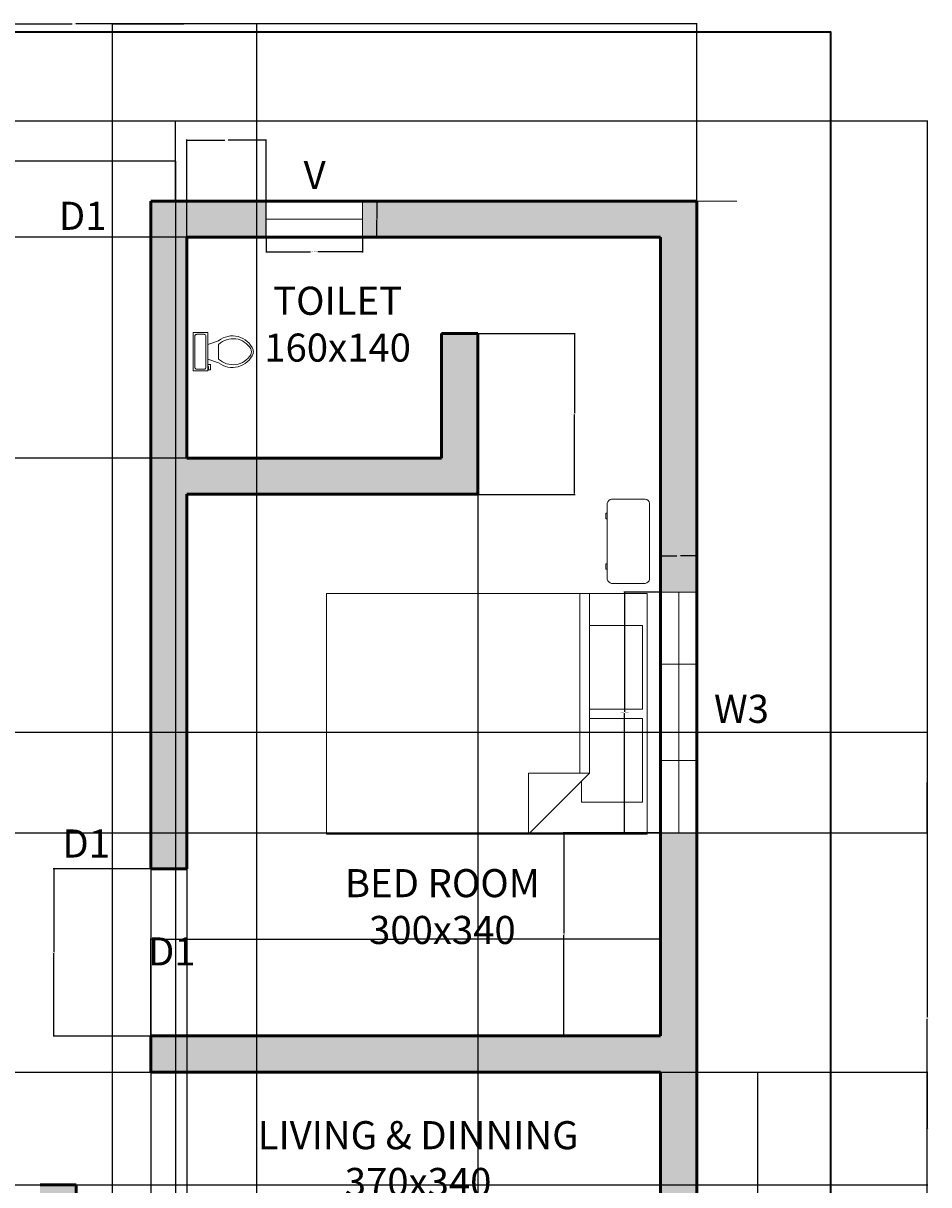
# Model space of a CAD drawing. Units: inches. Extents: x 5191 to 5616, y 7031 to 7539.
# Tile 4 of 4: x 5390 to 5616, y 7250 to 7539. Entities that reach past the tile are written whole.
import ezdxf

# ---------------------------------------------------------------- set-up
doc = ezdxf.new("R2010")
doc.units = ezdxf.units.IN
for name, color, linetype, lineweight in [('A-ANNO-DIMS', 2, 'Continuous', 13), ('A-ANNO-TEXT', 7, 'Continuous', 18), ('A-ANNO-TTLB', 7, 'Continuous', 35), ('A-AREA-IDEN', 7, 'Continuous', 25), ('A-FLOR-FIXT', 9, 'Continuous', 18), ('A-FLOR-STRS', 7, 'Continuous', 25), ('A-FURN', 8, 'Continuous', 18), ('A-GLAZ', 4, 'Continuous', 18), ('A-WALL', 7, 'Continuous', 50)]:
    doc.layers.add(name, color=color, linetype=linetype, lineweight=lineweight)
doc.layers.add('A-WALL-PATT', color=177, linetype='Continuous', lineweight=13, true_color=0x293189)
doc.styles.get("Standard").update_dxf_attribs({"font": 'arial.ttf'})
doc.dimstyles.get("Standard").update_dxf_attribs({"dimtxt": 0.18, "dimasz": 0.18, "dimexe": 0.18, "dimexo": 0.0625, "dimgap": 0.09, "dimtad": 0, "dimtih": 1, "dimtoh": 1, "dimdec": 4, "dimzin": 0, "dimdsep": 46, "dimtxsty": 'Standard', "dimcen": 0.09, "dimadec": 0, "dimazin": 0, "dimtfac": 1, "dimtdec": 4, "dimtofl": 0, "dimtmove": 0, "dimatfit": 3, "dimfxl": 1, "dimtolj": 1, "dimtzin": 0, "dimarcsym": 0})

# ---------------------------------------------------------------- blocks, each defined once
blk = doc.blocks.new('*U2')
for p, q in [((9.5, -6), (9.5, -2)), ((-10, -8.5), (-8, -8.5)), ((-10, -9.5), (-10, -8.5)), ((-7, -9.5), (-10, -9.5)), ((-8, -8.5), (-8, -8)), ((-7, -8), (-7, -9.5)), ((-4, -8), (-6, -14)), ((4, -8), (6, -14)), ((4, -14), (-4, -14))]:
    blk.add_line(p, q)
blk.add_lwpolyline([(10.5, -8), (10.5, 0), (-10.5, 0), (-10.5, -8)], close=True)
for points in [[(-9.5, -2), (-9.5, -6)], [(8.5, -1), (-8.5, -1)], [(-8.5, -7), (8.5, -7)]]:
    blk.add_lwpolyline(points)
for centre, radius, start, end in [((-8.62, -1.88), 0.884, 81.8699, 188.1301), ((-8.62, -6.12), 0.884, 171.8699, 278.1301), ((8.62, -1.88), 0.884, 351.8699, 98.1301), ((8.62, -6.12), 0.884, 261.8699, 8.1301), ((3.52, -21.58), 12.17, 141.46911, 247.97143), ((4.2, -21.82), 11.33, 136.36773, 238.94682), ((-3.52, -21.58), 12.17, 292.02843, 38.53071), ((-4.2, -21.82), 11.33, 301.05301, 43.63209), ((0, -27.88), 4, 245.73182, 294.26817), ((0, -29), 4, 254.86053, 285.13947)]:
    blk.add_arc(centre, radius, start, end)
blk = doc.blocks.new('Bed - Queen')
for p, q in [((0, -80.00003), (0, 0)), ((0, 0), (59.99999, 0)), ((59.99999, 0), (59.99999, -80.00003)), ((7.99999, -1.2), (28.79998, -1.2)), ((7.99999, -14.4), (7.99999, -1.2)), ((28.79998, -1.2), (28.79998, -14.4)), ((31.19999, -1.2), (51.99999, -1.2)), ((31.19999, -14.4), (31.19999, -1.2)), ((51.99999, -1.2), (51.99999, -16.4)), ((0, -14.4), (44.8, -14.4)), ((59.99999, -29.6), (44.8, -14.4)), ((44.8, -14.4), (44.8, -29.6)), ((44.8, -16.8), (0, -16.8)), ((51.99999, -16.4), (46.79936, -16.4)), ((44.8, -29.6), (59.99999, -29.6)), ((59.99999, -80.00003), (0, -80.00003))]:
    blk.add_line(p, q)
blk = doc.blocks.new('Desk - 30 x 60 in.')
for p, q in [((-26.999995, 0), (26.999995, 0)), ((-29.999995, -27), (-29.999995, -3)), ((29.999995, -3), (29.999995, -27)), ((26.999995, -30), (-26.999995, -30)), ((-20.000005, -30), (-20.000005, -31)), ((-20.000005, -31), (-16.000005, -31)), ((-16.000005, -31), (-16.000005, -30)), ((15.999995, -31), (15.999995, -30)), ((19.999995, -31), (15.999995, -31)), ((19.999995, -30), (19.999995, -31))]:
    blk.add_line(p, q)
for centre, start, end in [((-26.499995, -3.5), 98.1301, 171.8699), ((26.499995, -3.5), 8.130102, 81.8699), ((-26.499995, -26.5), 188.1301, 261.8699), ((26.499995, -26.5), 278.1301, 351.8699)]:
    blk.add_arc(centre, 3.535534, start, end)
blk = doc.blocks.new('WIN-W3-60IN')
for p, q in [((9, 60), (0, 60)), ((4.5, 60), (4.5, 0)), ((9, 42), (0, 42)), ((9, 18), (0, 18)), ((9, 0), (0, 0))]:
    blk.add_line(p, q)
blk = doc.blocks.new('VENT-24IN')
for p, q in [((0, 0), (0, 9)), ((24, 0), (24, 9)), ((0, 4.5), (24, 4.5))]:
    blk.add_line(p, q)
blk = doc.blocks.new('*D17')
at = {"layer": 'A-ANNO-DIMS', "color": 0, "lineweight": -2, "transparency": 16777216}
for p, q in [((5549.01, 7397.33), (5539.89, 7397.33)), ((5540.07, 7397.15), (5540.07, 7367.52)), ((5540.07, 7337.51), (5540.07, 7367.15)), ((5549.01, 7337.33), (5539.89, 7337.33))]:
    blk.add_line(p, q, dxfattribs=at)
at = {"layer": 'A-ANNO-DIMS', "color": 0, "transparency": 16777216}
for points in [[(5540.04, 7397.15), (5540.1, 7397.15), (5540.07, 7397.33)], [(5540.04, 7337.51), (5540.1, 7337.51), (5540.07, 7337.33)]]:
    blk.add_solid(points, dxfattribs=at)
at = {"layer": 'Defpoints', "color": 0, "transparency": 16777216}
for p in [(5540.07, 7397.33), (5549.07, 7397.33), (5549.07, 7337.33)]:
    blk.add_point(p, dxfattribs=at)
at = {"layer": 'A-ANNO-DIMS', "color": 0, "transparency": 16777216, "insert": (5540.07, 7367.33), "char_height": 0.18, "attachment_point": 5}
blk.add_mtext('\\A1;WINDOW W3 60 TYP.', dxfattribs=at)
blk = doc.blocks.new('*D18')
at = {"layer": 'A-ANNO-DIMS', "color": 0, "lineweight": -2, "transparency": 16777216}
for p, q in [((5549.07, 7397.4), (5549.07, 7406.51)), ((5549.25, 7406.33), (5553.11, 7406.33)), ((5557.89, 7406.33), (5554.03, 7406.33)), ((5558.07, 7397.4), (5558.07, 7406.51))]:
    blk.add_line(p, q, dxfattribs=at)
at = {"layer": 'A-ANNO-DIMS', "color": 0, "transparency": 16777216}
for points in [[(5549.25, 7406.36), (5549.25, 7406.3), (5549.07, 7406.33)], [(5557.89, 7406.36), (5557.89, 7406.3), (5558.07, 7406.33)]]:
    blk.add_solid(points, dxfattribs=at)
at = {"layer": 'Defpoints', "color": 0, "transparency": 16777216}
for p in [(5558.07, 7406.33), (5549.07, 7397.33), (5558.07, 7397.33)]:
    blk.add_point(p, dxfattribs=at)
at = {"layer": 'A-ANNO-DIMS', "color": 0, "transparency": 16777216, "insert": (5553.57, 7406.33), "char_height": 0.18, "attachment_point": 5}
blk.add_mtext('\\A1;9 TYP.', dxfattribs=at)
blk = doc.blocks.new('*D21')
at = {"layer": 'A-ANNO-DIMS', "color": 0, "lineweight": -2, "transparency": 16777216}
for p, q in [((5450.73, 7485.71), (5450.73, 7481.99)), ((5474.73, 7485.71), (5474.73, 7481.99)), ((5450.91, 7482.17), (5461.83, 7482.17)), ((5474.55, 7482.17), (5463.63, 7482.17))]:
    blk.add_line(p, q, dxfattribs=at)
at = {"layer": 'A-ANNO-DIMS', "color": 0, "transparency": 16777216}
for points in [[(5450.91, 7482.2), (5450.91, 7482.14), (5450.73, 7482.17)], [(5474.55, 7482.2), (5474.55, 7482.14), (5474.73, 7482.17)]]:
    blk.add_solid(points, dxfattribs=at)
at = {"layer": 'Defpoints', "color": 0, "transparency": 16777216}
for p in [(5450.73, 7485.77), (5474.73, 7485.77), (5474.73, 7482.17)]:
    blk.add_point(p, dxfattribs=at)
at = {"layer": 'A-ANNO-DIMS', "color": 0, "transparency": 16777216, "insert": (5462.73, 7482.17), "char_height": 0.18, "attachment_point": 5}
blk.add_mtext('\\A1;VENT 24 TYP.', dxfattribs=at)
blk = doc.blocks.new('*D22')
at = {"layer": 'A-ANNO-DIMS', "color": 0, "lineweight": -2, "transparency": 16777216}
for p, q in [((5474.79, 7494.77), (5478.51, 7494.77)), ((5478.33, 7494.59), (5478.33, 7490.46)), ((5478.33, 7485.95), (5478.33, 7490.09)), ((5474.79, 7485.77), (5478.51, 7485.77))]:
    blk.add_line(p, q, dxfattribs=at)
at = {"layer": 'A-ANNO-DIMS', "color": 0, "transparency": 16777216}
for points in [[(5478.3, 7494.59), (5478.36, 7494.59), (5478.33, 7494.77)], [(5478.3, 7485.95), (5478.36, 7485.95), (5478.33, 7485.77)]]:
    blk.add_solid(points, dxfattribs=at)
at = {"layer": 'Defpoints', "color": 0, "transparency": 16777216}
for p in [(5474.73, 7494.77), (5478.33, 7494.77), (5474.73, 7485.77)]:
    blk.add_point(p, dxfattribs=at)
at = {"layer": 'A-ANNO-DIMS', "color": 0, "transparency": 16777216, "insert": (5478.33, 7490.27), "char_height": 0.18, "attachment_point": 5}
blk.add_mtext('\\A1;9 TYP.', dxfattribs=at)
blk = doc.blocks.new('*D31')
at = {"layer": 'A-ANNO-DIMS', "color": 0, "lineweight": -2, "transparency": 16777216}
for p, q in [((5247.63, 7494.84), (5247.63, 7539.1)), ((5247.81, 7538.92), (5402.39, 7538.92)), ((5557.89, 7538.92), (5403.31, 7538.92)), ((5558.07, 7494.84), (5558.07, 7539.1))]:
    blk.add_line(p, q, dxfattribs=at)
at = {"layer": 'A-ANNO-DIMS', "color": 0, "transparency": 16777216}
for points in [[(5247.81, 7538.95), (5247.81, 7538.89), (5247.63, 7538.92)], [(5557.89, 7538.95), (5557.89, 7538.89), (5558.07, 7538.92)]]:
    blk.add_solid(points, dxfattribs=at)
at = {"layer": 'Defpoints', "color": 0, "transparency": 16777216}
for p in [(5558.07, 7538.92), (5247.63, 7494.77), (5558.07, 7494.77)]:
    blk.add_point(p, dxfattribs=at)
at = {"layer": 'A-ANNO-DIMS', "color": 0, "transparency": 16777216, "insert": (5402.85, 7538.92), "char_height": 0.18, "attachment_point": 5}
blk.add_mtext('\\A1;310.44', dxfattribs=at)
blk = doc.blocks.new('*D32')
at = {"layer": 'A-ANNO-DIMS', "color": 0, "lineweight": -2, "transparency": 16777216}
for p, q in [((5428.24, 7514.77), (5615.71, 7514.77)), ((5615.53, 7514.59), (5615.53, 7291.37)), ((5615.53, 7067.79), (5615.53, 7291.01)), ((5466.73, 7067.61), (5615.71, 7067.61))]:
    blk.add_line(p, q, dxfattribs=at)
at = {"layer": 'A-ANNO-DIMS', "color": 0, "transparency": 16777216}
for points in [[(5615.5, 7514.59), (5615.56, 7514.59), (5615.53, 7514.77)], [(5615.5, 7067.79), (5615.56, 7067.79), (5615.53, 7067.61)]]:
    blk.add_solid(points, dxfattribs=at)
at = {"layer": 'Defpoints', "color": 0, "transparency": 16777216}
for p in [(5428.18, 7514.77), (5615.53, 7514.77), (5466.67, 7067.61)]:
    blk.add_point(p, dxfattribs=at)
at = {"layer": 'A-ANNO-DIMS', "color": 0, "transparency": 16777216, "insert": (5615.53, 7291.19), "char_height": 0.18, "attachment_point": 5}
blk.add_mtext('\\A1;447.2', dxfattribs=at)
blk = doc.blocks.new('*D38')
at = {"layer": 'A-ANNO-DIMS', "color": 0, "lineweight": -2, "transparency": 16777216}
for p, q in [((5379.71, 7504.71), (5379.71, 7030.92)), ((5428.18, 7504.71), (5428.18, 7030.92)), ((5379.89, 7031.1), (5403.55, 7031.1)), ((5428, 7031.1), (5404.34, 7031.1))]:
    blk.add_line(p, q, dxfattribs=at)
at = {"layer": 'A-ANNO-DIMS', "color": 0, "transparency": 16777216}
for points in [[(5379.89, 7031.13), (5379.89, 7031.07), (5379.71, 7031.1)], [(5428, 7031.13), (5428, 7031.07), (5428.18, 7031.1)]]:
    blk.add_solid(points, dxfattribs=at)
at = {"layer": 'Defpoints', "color": 0, "transparency": 16777216}
for p in [(5379.71, 7504.77), (5428.18, 7504.77), (5428.18, 7031.1)]:
    blk.add_point(p, dxfattribs=at)
at = {"layer": 'A-ANNO-DIMS', "color": 0, "transparency": 16777216, "insert": (5403.95, 7031.1), "char_height": 0.18, "attachment_point": 5}
blk.add_mtext('\\A1;48.47', dxfattribs=at)
blk = doc.blocks.new('*D44')
at = {"layer": 'A-ANNO-DIMS', "color": 0, "lineweight": -2, "transparency": 16777216}
for p, q in [((5549.13, 7277.69), (5573.4, 7277.69)), ((5573.22, 7277.51), (5573.22, 7210.98)), ((5573.22, 7144.07), (5573.22, 7210.61)), ((5549.13, 7143.89), (5573.4, 7143.89))]:
    blk.add_line(p, q, dxfattribs=at)
at = {"layer": 'A-ANNO-DIMS', "color": 0, "transparency": 16777216}
for points in [[(5573.19, 7277.51), (5573.25, 7277.51), (5573.22, 7277.69)], [(5573.19, 7144.07), (5573.25, 7144.07), (5573.22, 7143.89)]]:
    blk.add_solid(points, dxfattribs=at)
at = {"layer": 'Defpoints', "color": 0, "transparency": 16777216}
for p in [(5549.07, 7277.69), (5549.07, 7143.89), (5573.22, 7143.89)]:
    blk.add_point(p, dxfattribs=at)
at = {"layer": 'A-ANNO-DIMS', "color": 0, "transparency": 16777216, "insert": (5573.22, 7210.79), "char_height": 0.18, "attachment_point": 5}
blk.add_mtext('\\A1;133.8', dxfattribs=at)
blk = doc.blocks.new('*D45')
at = {"layer": 'A-ANNO-DIMS', "color": 0, "lineweight": -2, "transparency": 16777216}
for p, q in [((5421.99, 7286.76), (5421.99, 7311.02)), ((5422.17, 7310.84), (5485.08, 7310.84)), ((5548.89, 7310.84), (5485.99, 7310.84)), ((5549.07, 7286.76), (5549.07, 7311.02))]:
    blk.add_line(p, q, dxfattribs=at)
at = {"layer": 'A-ANNO-DIMS', "color": 0, "transparency": 16777216}
for points in [[(5422.17, 7310.87), (5422.17, 7310.81), (5421.99, 7310.84)], [(5548.89, 7310.87), (5548.89, 7310.81), (5549.07, 7310.84)]]:
    blk.add_solid(points, dxfattribs=at)
at = {"layer": 'Defpoints', "color": 0, "transparency": 16777216}
for p in [(5549.07, 7310.84), (5421.99, 7286.69), (5549.07, 7286.69)]:
    blk.add_point(p, dxfattribs=at)
at = {"layer": 'A-ANNO-DIMS', "color": 0, "transparency": 16777216, "insert": (5485.53, 7310.84), "char_height": 0.18, "attachment_point": 5}
blk.add_mtext('\\A1;127.08', dxfattribs=at)
blk = doc.blocks.new('*D46')
at = {"layer": 'A-ANNO-DIMS', "color": 0, "lineweight": -2, "transparency": 16777216}
for p, q in [((5549.01, 7337.33), (5524.74, 7337.33)), ((5524.92, 7337.15), (5524.92, 7312.2)), ((5524.92, 7286.87), (5524.92, 7311.83)), ((5549.01, 7286.69), (5524.74, 7286.69))]:
    blk.add_line(p, q, dxfattribs=at)
at = {"layer": 'A-ANNO-DIMS', "color": 0, "transparency": 16777216}
for points in [[(5524.89, 7337.15), (5524.95, 7337.15), (5524.92, 7337.33)], [(5524.89, 7286.87), (5524.95, 7286.87), (5524.92, 7286.69)]]:
    blk.add_solid(points, dxfattribs=at)
at = {"layer": 'Defpoints', "color": 0, "transparency": 16777216}
for p in [(5524.92, 7337.33), (5549.07, 7337.33), (5549.07, 7286.69)]:
    blk.add_point(p, dxfattribs=at)
at = {"layer": 'A-ANNO-DIMS', "color": 0, "transparency": 16777216, "insert": (5524.92, 7312.01), "char_height": 0.18, "attachment_point": 5}
blk.add_mtext('\\A1;50.64', dxfattribs=at)
blk = doc.blocks.new('*D49')
at = {"layer": 'A-ANNO-DIMS', "color": 0, "lineweight": -2, "transparency": 16777216}
for p, q in [((5385.99, 7494.71), (5385.99, 7030.92)), ((5421.99, 7494.71), (5421.99, 7030.92)), ((5386.17, 7031.1), (5403.77, 7031.1)), ((5421.81, 7031.1), (5404.21, 7031.1))]:
    blk.add_line(p, q, dxfattribs=at)
at = {"layer": 'A-ANNO-DIMS', "color": 0, "transparency": 16777216}
for points in [[(5386.17, 7031.13), (5386.17, 7031.07), (5385.99, 7031.1)], [(5421.81, 7031.13), (5421.81, 7031.07), (5421.99, 7031.1)]]:
    blk.add_solid(points, dxfattribs=at)
at = {"layer": 'Defpoints', "color": 0, "transparency": 16777216}
for p in [(5385.99, 7494.77), (5421.99, 7494.77), (5421.99, 7031.1)]:
    blk.add_point(p, dxfattribs=at)
at = {"layer": 'A-ANNO-DIMS', "color": 0, "transparency": 16777216, "insert": (5403.99, 7031.1), "char_height": 0.18, "attachment_point": 5}
blk.add_mtext('\\A1;36', dxfattribs=at)
blk = doc.blocks.new('*D50')
at = {"layer": 'A-ANNO-DIMS', "color": 0, "lineweight": -2, "transparency": 16777216}
for p, q in [((5430.99, 7485.84), (5430.99, 7510.1)), ((5431.17, 7509.92), (5440.48, 7509.92)), ((5450.55, 7509.92), (5441.25, 7509.92)), ((5450.73, 7485.84), (5450.73, 7510.1))]:
    blk.add_line(p, q, dxfattribs=at)
at = {"layer": 'A-ANNO-DIMS', "color": 0, "transparency": 16777216}
for points in [[(5431.17, 7509.95), (5431.17, 7509.89), (5430.99, 7509.92)], [(5450.55, 7509.95), (5450.55, 7509.89), (5450.73, 7509.92)]]:
    blk.add_solid(points, dxfattribs=at)
at = {"layer": 'Defpoints', "color": 0, "transparency": 16777216}
for p in [(5450.73, 7509.92), (5430.99, 7485.77), (5450.73, 7485.77)]:
    blk.add_point(p, dxfattribs=at)
at = {"layer": 'A-ANNO-DIMS', "color": 0, "transparency": 16777216, "insert": (5440.86, 7509.92), "char_height": 0.18, "attachment_point": 5}
blk.add_mtext('\\A1;19.74', dxfattribs=at)
blk = doc.blocks.new('*D51')
at = {"layer": 'A-ANNO-DIMS', "color": 0, "lineweight": -2, "transparency": 16777216}
for p, q in [((5412.46, 7143.96), (5412.46, 7539.1)), ((5412.64, 7538.92), (5430.24, 7538.92)), ((5448.28, 7538.92), (5430.68, 7538.92)), ((5448.46, 7143.96), (5448.46, 7539.1))]:
    blk.add_line(p, q, dxfattribs=at)
at = {"layer": 'A-ANNO-DIMS', "color": 0, "transparency": 16777216}
for points in [[(5412.64, 7538.95), (5412.64, 7538.89), (5412.46, 7538.92)], [(5448.28, 7538.95), (5448.28, 7538.89), (5448.46, 7538.92)]]:
    blk.add_solid(points, dxfattribs=at)
at = {"layer": 'Defpoints', "color": 0, "transparency": 16777216}
for p in [(5448.46, 7538.92), (5412.46, 7143.89), (5448.46, 7143.89)]:
    blk.add_point(p, dxfattribs=at)
at = {"layer": 'A-ANNO-DIMS', "color": 0, "transparency": 16777216, "insert": (5430.46, 7538.92), "char_height": 0.18, "attachment_point": 5}
blk.add_mtext('\\A1;36', dxfattribs=at)
blk = doc.blocks.new('*D54')
at = {"layer": 'A-ANNO-DIMS', "color": 0, "lineweight": -2, "transparency": 16777216}
for p, q in [((5430.99, 7421.63), (5430.99, 7030.92)), ((5503.47, 7421.63), (5503.47, 7030.92)), ((5431.17, 7031.1), (5466.84, 7031.1)), ((5503.29, 7031.1), (5467.62, 7031.1))]:
    blk.add_line(p, q, dxfattribs=at)
at = {"layer": 'A-ANNO-DIMS', "color": 0, "transparency": 16777216}
for points in [[(5431.17, 7031.13), (5431.17, 7031.07), (5430.99, 7031.1)], [(5503.29, 7031.13), (5503.29, 7031.07), (5503.47, 7031.1)]]:
    blk.add_solid(points, dxfattribs=at)
at = {"layer": 'Defpoints', "color": 0, "transparency": 16777216}
for p in [(5430.99, 7421.69), (5503.47, 7421.69), (5503.47, 7031.1)]:
    blk.add_point(p, dxfattribs=at)
at = {"layer": 'A-ANNO-DIMS', "color": 0, "transparency": 16777216, "insert": (5467.23, 7031.1), "char_height": 0.18, "attachment_point": 5}
blk.add_mtext('\\A1;72.48', dxfattribs=at)
blk = doc.blocks.new('*D55')
at = {"layer": 'A-ANNO-DIMS', "color": 0, "lineweight": -2, "transparency": 16777216}
for p, q in [((5430.93, 7485.77), (5191.41, 7485.77)), ((5191.59, 7485.59), (5191.59, 7458.42)), ((5191.59, 7430.87), (5191.59, 7458.05)), ((5430.93, 7430.69), (5191.41, 7430.69))]:
    blk.add_line(p, q, dxfattribs=at)
at = {"layer": 'A-ANNO-DIMS', "color": 0, "transparency": 16777216}
for points in [[(5191.56, 7485.59), (5191.62, 7485.59), (5191.59, 7485.77)], [(5191.56, 7430.87), (5191.62, 7430.87), (5191.59, 7430.69)]]:
    blk.add_solid(points, dxfattribs=at)
at = {"layer": 'Defpoints', "color": 0, "transparency": 16777216}
for p in [(5191.59, 7485.77), (5430.99, 7485.77), (5430.99, 7430.69)]:
    blk.add_point(p, dxfattribs=at)
at = {"layer": 'A-ANNO-DIMS', "color": 0, "transparency": 16777216, "insert": (5191.59, 7458.23), "char_height": 0.18, "attachment_point": 5}
blk.add_mtext('\\A1;55.08', dxfattribs=at)
blk = doc.blocks.new('*D60')
at = {"layer": 'A-ANNO-DIMS', "color": 0, "lineweight": -2, "transparency": 16777216}
for p, q in [((5343.97, 7277.69), (5615.71, 7277.69)), ((5615.53, 7277.51), (5615.53, 7263.84)), ((5615.53, 7249.79), (5615.53, 7263.47)), ((5343.97, 7249.61), (5615.71, 7249.61))]:
    blk.add_line(p, q, dxfattribs=at)
at = {"layer": 'A-ANNO-DIMS', "color": 0, "transparency": 16777216}
for points in [[(5615.5, 7277.51), (5615.56, 7277.51), (5615.53, 7277.69)], [(5615.5, 7249.79), (5615.56, 7249.79), (5615.53, 7249.61)]]:
    blk.add_solid(points, dxfattribs=at)
at = {"layer": 'Defpoints', "color": 0, "transparency": 16777216}
for p in [(5343.91, 7277.69), (5615.53, 7277.69), (5343.91, 7249.61)]:
    blk.add_point(p, dxfattribs=at)
at = {"layer": 'A-ANNO-DIMS', "color": 0, "transparency": 16777216, "insert": (5615.53, 7263.65), "char_height": 0.18, "attachment_point": 5}
blk.add_mtext('\\A1;28.08', dxfattribs=at)
blk = doc.blocks.new('*D62')
at = {"layer": 'A-ANNO-DIMS', "color": 0, "lineweight": -2, "transparency": 16777216}
for p, q in [((5361.85, 7362.43), (5615.71, 7362.43)), ((5615.53, 7362.25), (5615.53, 7350.06)), ((5615.53, 7337.51), (5615.53, 7349.7)), ((5361.85, 7337.33), (5615.71, 7337.33))]:
    blk.add_line(p, q, dxfattribs=at)
at = {"layer": 'A-ANNO-DIMS', "color": 0, "transparency": 16777216}
for points in [[(5615.5, 7362.25), (5615.56, 7362.25), (5615.53, 7362.43)], [(5615.5, 7337.51), (5615.56, 7337.51), (5615.53, 7337.33)]]:
    blk.add_solid(points, dxfattribs=at)
at = {"layer": 'Defpoints', "color": 0, "transparency": 16777216}
for p in [(5361.78, 7362.43), (5615.53, 7362.43), (5361.78, 7337.33)]:
    blk.add_point(p, dxfattribs=at)
at = {"layer": 'A-ANNO-DIMS', "color": 0, "transparency": 16777216, "insert": (5615.53, 7349.88), "char_height": 0.18, "attachment_point": 5}
blk.add_mtext('\\A1;25.094', dxfattribs=at)
blk = doc.blocks.new('*D65')
at = {"layer": 'A-ANNO-DIMS', "color": 0, "lineweight": -2, "transparency": 16777216}
for p, q in [((5421.93, 7328.33), (5397.66, 7328.33)), ((5397.84, 7328.15), (5397.84, 7307.7)), ((5397.84, 7286.87), (5397.84, 7307.33)), ((5421.93, 7286.69), (5397.66, 7286.69))]:
    blk.add_line(p, q, dxfattribs=at)
at = {"layer": 'A-ANNO-DIMS', "color": 0, "transparency": 16777216}
for points in [[(5397.81, 7328.15), (5397.87, 7328.15), (5397.84, 7328.33)], [(5397.81, 7286.87), (5397.87, 7286.87), (5397.84, 7286.69)]]:
    blk.add_solid(points, dxfattribs=at)
at = {"layer": 'Defpoints', "color": 0, "transparency": 16777216}
for p in [(5397.84, 7328.33), (5421.99, 7328.33), (5421.99, 7286.69)]:
    blk.add_point(p, dxfattribs=at)
at = {"layer": 'A-ANNO-DIMS', "color": 0, "transparency": 16777216, "insert": (5397.84, 7307.51), "char_height": 0.18, "attachment_point": 5}
blk.add_mtext('\\A1;41.64', dxfattribs=at)
blk = doc.blocks.new('*D66')
at = {"layer": 'A-ANNO-DIMS', "color": 0, "lineweight": -2, "transparency": 16777216}
for p, q in [((5503.53, 7461.77), (5527.8, 7461.77)), ((5527.62, 7461.59), (5527.62, 7441.92)), ((5527.62, 7421.87), (5527.62, 7441.55)), ((5503.53, 7421.69), (5527.8, 7421.69))]:
    blk.add_line(p, q, dxfattribs=at)
at = {"layer": 'A-ANNO-DIMS', "color": 0, "transparency": 16777216}
for points in [[(5527.59, 7461.59), (5527.65, 7461.59), (5527.62, 7461.77)], [(5527.59, 7421.87), (5527.65, 7421.87), (5527.62, 7421.69)]]:
    blk.add_solid(points, dxfattribs=at)
at = {"layer": 'Defpoints', "color": 0, "transparency": 16777216}
for p in [(5503.47, 7461.77), (5503.47, 7421.69), (5527.62, 7421.69)]:
    blk.add_point(p, dxfattribs=at)
at = {"layer": 'A-ANNO-DIMS', "color": 0, "transparency": 16777216, "insert": (5527.62, 7441.73), "char_height": 0.18, "attachment_point": 5}
blk.add_mtext('\\A1;40.08', dxfattribs=at)

msp = doc.modelspace()

# ---------------------------------------------------------------- hatches: boundary and pattern name
at = {"layer": 'A-WALL-PATT'}
h = msp.add_hatch(color=256, dxfattribs=at)
h.dxf.hatch_style = 1
h.paths.add_polyline_path([(5297.311, 7494.7733), (5247.631, 7494.7733), (5247.631, 7441.5533), (5256.631, 7441.5533), (5256.631, 7485.7733), (5297.311, 7485.7733)])
h.paths.add_polyline_path([(5503.471, 7430.6933), (5503.471, 7461.7733), (5494.471, 7461.7733), (5494.471, 7430.6933), (5430.991, 7430.6933), (5430.991, 7485.7733), (5450.731, 7485.7733), (5450.731, 7494.7733), (5421.991, 7494.7733), (5421.991, 7485.7733), (5421.991, 7337.3333), (5421.991, 7328.3333), (5430.991, 7328.3333), (5430.991, 7337.3333), (5430.991, 7421.6933), (5503.471, 7421.6933)])
h.paths.add_polyline_path([(5385.991, 7494.7733), (5345.311, 7494.7733), (5345.311, 7485.7733), (5385.991, 7485.7733)])
h.paths.add_polyline_path([(5558.071, 7494.7733), (5474.731, 7494.7733), (5474.731, 7485.7733), (5494.471, 7485.7733), (5503.471, 7485.7733), (5549.071, 7485.7733), (5549.071, 7397.3333), (5558.071, 7397.3333)])
h.paths.add_polyline_path([(5385.991, 7337.3333), (5256.631, 7337.3333), (5256.631, 7381.5533), (5247.631, 7381.5533), (5247.631, 7337.3333), (5247.631, 7328.3333), (5247.631, 7300.9733), (5256.631, 7300.9733), (5256.631, 7328.3333), (5385.991, 7328.3333)])
h.paths.add_polyline_path([(5358.391, 7249.6133), (5303.911, 7249.6133), (5256.631, 7249.6133), (5256.631, 7276.9733), (5247.631, 7276.9733), (5247.631, 7249.6133), (5247.631, 7240.6133), (5247.631, 7207.6133), (5256.631, 7207.6133), (5256.631, 7240.6133), (5303.911, 7240.6133), (5358.391, 7240.6133)])
h.paths.add_polyline_path([(5256.631, 7114.6133), (5256.631, 7147.6133), (5247.631, 7147.6133), (5247.631, 7114.6133), (5247.631, 7105.6133), (5247.631, 7087.6133), (5301.511, 7087.6133), (5301.511, 7096.6133), (5256.631, 7096.6133)])
h.paths.add_polyline_path([(5403.391, 7105.6133), (5403.391, 7114.6133), (5403.391, 7134.8933), (5412.4598, 7134.8933), (5412.4598, 7143.8933), (5403.391, 7143.8933), (5403.391, 7249.6133), (5394.391, 7249.6133), (5394.391, 7143.8933), (5394.391, 7134.8933), (5394.391, 7114.6133), (5394.391, 7096.6133), (5349.511, 7096.6133), (5349.511, 7087.6133), (5403.391, 7087.6133)])
h.paths.add_polyline_path([(5558.071, 7143.8933), (5558.071, 7186.7933), (5549.071, 7186.7933), (5549.071, 7143.8933), (5527.2654, 7143.8933), (5527.2654, 7134.8933), (5558.071, 7134.8933)])
h.paths.add_polyline_path([(5479.2654, 7143.8933), (5448.4598, 7143.8933), (5448.4598, 7134.8933), (5479.2654, 7134.8933)])
h.paths.add_polyline_path([(5558.071, 7337.3333), (5549.071, 7337.3333), (5549.071, 7286.6933), (5421.991, 7286.6933), (5421.991, 7277.6933), (5430.991, 7277.6933), (5549.071, 7277.6933), (5549.071, 7234.7933), (5558.071, 7234.7933), (5558.071, 7277.6933)])

# ---------------------------------------------------------------- linework, layer by layer
at = {"layer": 'A-ANNO-DIMS'}
for q in [(5558.071, 7504.7733), (5568.071, 7494.7733)]:
    msp.add_line((5558.071, 7494.7733), q, dxfattribs=at)
at = {"layer": 'A-ANNO-TTLB'}
msp.add_lwpolyline([(5215.7388, 7536.9841), (5591.3795, 7536.9841), (5591.3795, 7055.2452), (5215.7388, 7055.2452)], close=True, dxfattribs=at)
at = {"layer": 'A-FLOR-STRS'}
for p, q in [((5379.7136, 7514.7733), (5428.1805, 7514.7733)), ((5428.1805, 7494.7733), (5428.1805, 7514.7733)), ((5379.7136, 7504.7733), (5428.1805, 7504.7733))]:
    msp.add_line(p, q, dxfattribs=at)
at = {"layer": 'A-GLAZ'}
msp.add_line((5549.071, 7397.3333), (5549.071, 7337.3333), dxfattribs=at)
at = {"layer": 'A-WALL'}
for p, q in [((5421.991, 7485.7733), (5421.991, 7494.7733)), ((5421.991, 7494.7733), (5558.071, 7494.7733)), ((5558.071, 7494.7733), (5558.071, 7337.3333)), ((5421.991, 7485.7733), (5421.991, 7337.3333)), ((5430.991, 7485.7733), (5430.991, 7430.6933)), ((5430.991, 7485.7733), (5494.471, 7485.7733)), ((5494.471, 7485.7733), (5503.471, 7485.7733)), ((5503.471, 7485.7733), (5549.071, 7485.7733)), ((5549.071, 7485.7733), (5549.071, 7337.3333)), ((5494.471, 7461.7733), (5494.471, 7430.6933)), ((5494.471, 7461.7733), (5503.471, 7461.7733)), ((5503.471, 7461.7733), (5503.471, 7430.6933)), ((5430.991, 7430.6933), (5494.471, 7430.6933)), ((5503.471, 7430.6933), (5503.471, 7421.6933)), ((5430.991, 7421.6933), (5503.471, 7421.6933)), ((5430.991, 7421.6933), (5430.991, 7337.3333)), ((5421.991, 7337.3333), (5421.991, 7328.3333)), ((5430.991, 7337.3333), (5430.991, 7328.3333)), ((5549.071, 7337.3333), (5549.071, 7286.6933)), ((5558.071, 7337.3333), (5558.071, 7277.6933)), ((5421.991, 7328.3333), (5430.991, 7328.3333)), ((5421.991, 7286.6933), (5549.071, 7286.6933)), ((5421.991, 7286.6933), (5421.991, 7277.6933)), ((5430.991, 7277.6933), (5421.991, 7277.6933)), ((5430.991, 7277.6933), (5549.071, 7277.6933)), ((5549.071, 7277.6933), (5549.071, 7143.8933)), ((5558.071, 7277.6933), (5558.071, 7143.8933)), ((5394.391, 7249.6133), (5403.391, 7249.6133)), ((5403.391, 7249.6133), (5403.391, 7143.8933))]:
    msp.add_line(p, q, dxfattribs=at)

# ---------------------------------------------------------------- block references
at = {"layer": 'A-FLOR-FIXT', "xscale": 0.4558429364465041, "yscale": 0.4558429364465041, "zscale": 0.4558429364465041, "rotation": 90}
msp.add_blockref('*U2', (5432.5183, 7457.2373), dxfattribs=at)
at = {"layer": 'A-FURN', "xscale": 0.350301795417789, "yscale": 0.350301795417789, "zscale": 0.350301795417789, "rotation": 270}
msp.add_blockref('Desk - 30 x 60 in.', (5546.2909, 7410.0149), dxfattribs=at)
at = {"layer": 'A-FURN', "rotation": 270}
msp.add_blockref('Bed - Queen', (5545.7485, 7396.9827), dxfattribs=at)
at = {"layer": 'A-GLAZ'}
for name, p in [('VENT-24IN', (5450.731, 7485.773)), ('WIN-W3-60IN', (5549.071, 7337.333))]:
    msp.add_blockref(name, p, dxfattribs=at)

# ---------------------------------------------------------------- texts
at = {"layer": 'A-ANNO-TEXT', "char_height": 7, "attachment_point": 1}
for s, width, insert in [('\\pxqc;V', 29.703042, (5447.9778, 7504.7663)), ('\\pxqc;D1', 16.947643, (5396.5294, 7494.6114)), ('\\pxqc;W3', 29.703042, (5554.3709, 7371.7303)), ('\\pxqc;D1', 18.543886, (5396.6224, 7338.166)), ('\\pxqc;D1', 18.543886, (5417.9596, 7311.2676))]:
    msp.add_mtext_dynamic_manual_height_columns(s, width=width, gutter_width=12.5, heights=[0], dxfattribs=dict(at, insert=insert))
at = {"layer": 'A-AREA-IDEN', "char_height": 7, "attachment_point": 1}
for s, width, insert in [('\\pxqc;{\\fArial|b1|i0|c0|p34;TOILET\\P160x140}', 45.986288, (5445.562, 7473.4317)), ('\\pxqc;{\\fArial|b1|i0|c0|p34;BED ROOM\\P300x340}', 84.025987, (5452.6555, 7328.2856)), ('\\pxqc;{\\fArial|b1|i0|c0|p34;LIVING & DINNING\\P370x340}', 103.767041, (5436.7343, 7265.4722))]:
    msp.add_mtext_dynamic_manual_height_columns(s, width=width, gutter_width=12.5, heights=[0], dxfattribs=dict(at, insert=insert))

# ---------------------------------------------------------------- dimensions: what is measured, and where the dimension line sits
at = {"layer": 'A-ANNO-DIMS'}
for base, p1, p2, override, picture, middle in [((5558.071, 7538.9233), (5247.631, 7494.7733), (5558.071, 7494.7733), {"dimdec": 2, "dimlfac": 1, "dimrnd": 0, "dimzin": 0, "dimdsep": 46, "dimlunit": 2}, '*D31', (5402.851, 7538.9233)), ((5448.4598, 7538.9233), (5412.4598, 7143.8933), (5448.4598, 7143.8933), {"dimdec": 0, "dimlfac": 1, "dimrnd": 0, "dimzin": 0, "dimdsep": 46, "dimlunit": 2}, '*D51', (5430.4598, 7538.9233)), ((5428.1805, 7031.0952), (5379.7136, 7504.7733), (5428.1805, 7504.7733), {"dimdec": 2, "dimlfac": 1, "dimrnd": 0, "dimzin": 0, "dimdsep": 46, "dimlunit": 2}, '*D38', (5403.947, 7031.0952)), ((5421.991, 7031.0952), (5385.991, 7494.7733), (5421.991, 7494.7733), {"dimdec": 0, "dimlfac": 1, "dimrnd": 0, "dimzin": 0, "dimdsep": 46, "dimlunit": 2}, '*D49', (5403.991, 7031.0952)), ((5503.471, 7031.0952), (5430.991, 7421.6933), (5503.471, 7421.6933), {"dimdec": 2, "dimlfac": 1, "dimrnd": 0, "dimzin": 0, "dimdsep": 46, "dimlunit": 2}, '*D54', (5467.231, 7031.0952))]:
    dim = msp.add_linear_dim(base=base, p1=p1, p2=p2, dimstyle='Standard', override=override, dxfattribs=at)
    dim.commit()
    dim.dimension.update_dxf_attribs({"geometry": picture, "text_midpoint": middle})
for base, p1, p2, angle, override, picture, middle in [((5615.5295, 7514.7733), (5466.6673, 7067.6133), (5428.1805, 7514.7733), 90, {"dimdec": 1, "dimlfac": 1, "dimrnd": 0, "dimzin": 0, "dimdsep": 46, "dimlunit": 2}, '*D32', (5615.5295, 7291.1933)), ((5450.731, 7509.9233), (5430.991, 7485.7733), (5450.731, 7485.7733), 0, {"dimdec": 2, "dimlfac": 1, "dimrnd": 0, "dimzin": 0, "dimdsep": 46, "dimlunit": 2}, '*D50', (5440.861, 7509.9233)), ((5191.5888, 7485.7733), (5430.991, 7430.6933), (5430.991, 7485.7733), 90, {"dimdec": 2, "dimlfac": 1, "dimrnd": 0, "dimzin": 0, "dimdsep": 46, "dimlunit": 2}, '*D55', (5191.5888, 7458.2333)), ((5527.621, 7421.6933), (5503.471, 7461.7733), (5503.471, 7421.6933), 270, {"dimdec": 2, "dimlfac": 1, "dimrnd": 0, "dimzin": 0, "dimdsep": 46, "dimlunit": 2}, '*D66', (5527.621, 7441.7333)), ((5615.5295, 7362.4276), (5361.7831, 7337.3333), (5361.7831, 7362.4276), 90, {"dimdec": 3, "dimlfac": 1, "dimrnd": 0, "dimzin": 0, "dimdsep": 46, "dimlunit": 2}, '*D62', (5615.5295, 7349.8805)), ((5524.921, 7337.3333), (5549.071, 7286.6933), (5549.071, 7337.3333), 90, {"dimdec": 2, "dimlfac": 1, "dimrnd": 0, "dimzin": 0, "dimdsep": 46, "dimlunit": 2}, '*D46', (5524.921, 7312.0133)), ((5397.841, 7328.3333), (5421.991, 7286.6933), (5421.991, 7328.3333), 90, {"dimdec": 2, "dimlfac": 1, "dimrnd": 0, "dimzin": 0, "dimdsep": 46, "dimlunit": 2}, '*D65', (5397.841, 7307.5133)), ((5549.071, 7310.8433), (5421.991, 7286.6933), (5549.071, 7286.6933), 0, {"dimdec": 2, "dimlfac": 1, "dimrnd": 0, "dimzin": 0, "dimdsep": 46, "dimlunit": 2}, '*D45', (5485.531, 7310.8433)), ((5615.5295, 7277.6933), (5343.911, 7249.6133), (5343.911, 7277.6933), 90, {"dimdec": 2, "dimlfac": 1, "dimrnd": 0, "dimzin": 0, "dimdsep": 46, "dimlunit": 2}, '*D60', (5615.5295, 7263.6533)), ((5573.221, 7143.8933), (5549.071, 7277.6933), (5549.071, 7143.8933), 270, {"dimdec": 1, "dimlfac": 1, "dimrnd": 0, "dimzin": 0, "dimdsep": 46, "dimlunit": 2}, '*D44', (5573.221, 7210.7933))]:
    dim = msp.add_linear_dim(base=base, p1=p1, p2=p2, angle=angle, dimstyle='Standard', override=override, dxfattribs=at)
    dim.commit()
    dim.dimension.update_dxf_attribs({"geometry": picture, "text_midpoint": middle})
for base, p1, p2, text, picture, middle in [((5478.331, 7494.7733), (5474.731, 7485.7733), (5474.731, 7494.7733), '<> TYP.', '*D22', (5478.331, 7490.2733)), ((5540.071, 7397.3333), (5549.071, 7337.3333), (5549.071, 7397.3333), 'WINDOW W3 <> TYP.', '*D17', (5540.071, 7367.3333))]:
    dim = msp.add_linear_dim(base=base, p1=p1, p2=p2, angle=90, text=text, dimstyle='Standard', override={"dimdec": 0, "dimlfac": 1, "dimrnd": 0, "dimzin": 0, "dimdsep": 46, "dimlunit": 2}, dxfattribs=at)
    dim.commit()
    dim.dimension.update_dxf_attribs({"geometry": picture, "text_midpoint": middle})
for base, p1, p2, text, picture, middle in [((5474.731, 7482.1733), (5450.731, 7485.7733), (5474.731, 7485.7733), 'VENT <> TYP.', '*D21', (5462.731, 7482.1733)), ((5558.071, 7406.3333), (5549.071, 7397.3333), (5558.071, 7397.3333), '<> TYP.', '*D18', (5553.571, 7406.3333))]:
    dim = msp.add_linear_dim(base=base, p1=p1, p2=p2, text=text, dimstyle='Standard', override={"dimdec": 0, "dimlfac": 1, "dimrnd": 0, "dimzin": 0, "dimdsep": 46, "dimlunit": 2}, dxfattribs=at)
    dim.commit()
    dim.dimension.update_dxf_attribs({"geometry": picture, "text_midpoint": middle})

doc.saveas('drawing.dxf')
